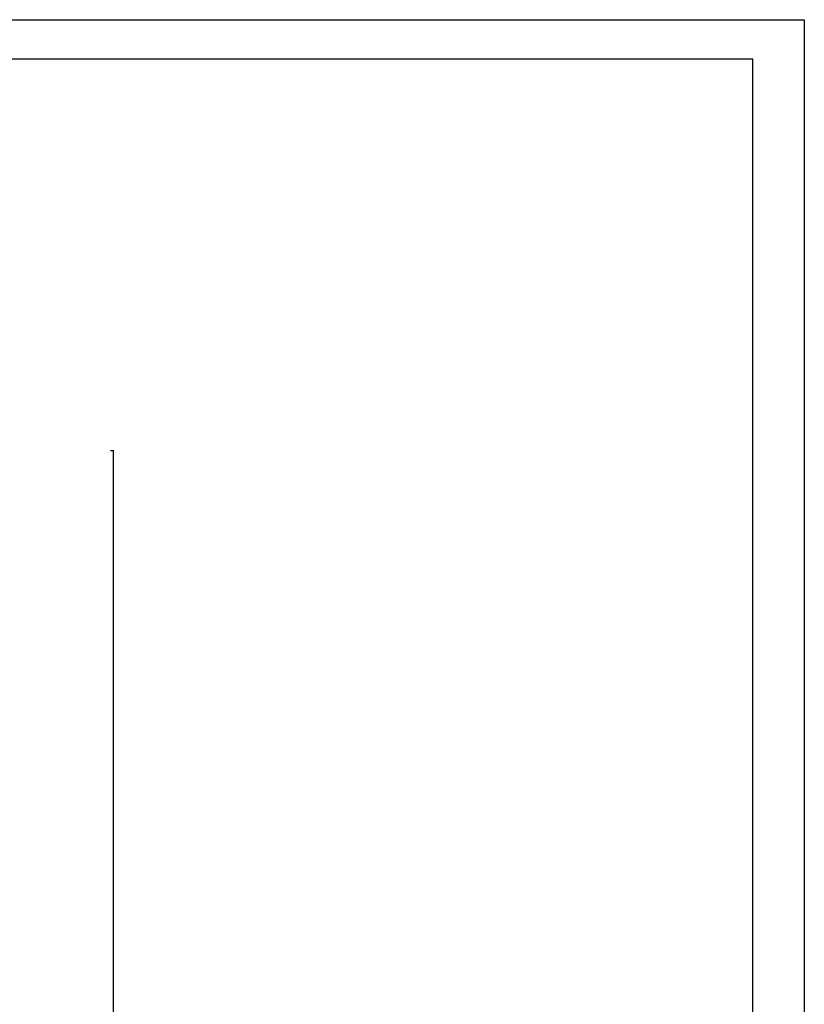
# Model space of a CAD drawing. Units: inches. Extents: x 0 to 4258, y 0 to 3769.
# Tile 30 of 30: x 4054 to 4258, y 3513 to 3769. Entities that reach past the tile are written whole.
import ezdxf

# ---------------------------------------------------------------- set-up
doc = ezdxf.new("R2010")
doc.units = ezdxf.units.IN
doc.header["$MEASUREMENT"] = 0
doc.layers.add('A-ANNO-DIMS', color=250, linetype='Continuous', lineweight=18)
doc.layers.add('A-ANNO-TTLB', color=250, linetype='Continuous', lineweight=25)
doc.styles.get("Standard").update_dxf_attribs({"font": 'arial.ttf'})
doc.dimstyles.get("Standard").update_dxf_attribs({"dimtxt": 7, "dimasz": 0.18, "dimexe": 0.18, "dimexo": 0.0625, "dimgap": 0.09, "dimtad": 0, "dimtih": 1, "dimtoh": 1, "dimzin": 0, "dimdsep": 46, "dimlunit": 3, "dimtxsty": 'Standard', "dimcen": 0.09, "dimadec": 0, "dimazin": 0, "dimtfac": 1, "dimtofl": 0, "dimtmove": 0, "dimatfit": 3, "dimfxl": 1, "dimtolj": 1, "dimtzin": 0, "dimarcsym": 0})

# ---------------------------------------------------------------- blocks, each defined once
blk = doc.blocks.new('*D26')
at = {"layer": 'A-ANNO-DIMS', "color": 0, "lineweight": -2, "transparency": 16777216}
for p, q in [((4077.41, 3656.79), (4078.27, 3656.79)), ((4078.09, 3656.61), (4078.09, 3329.69)), ((4078.09, 2995.47), (4078.09, 3322.39)), ((4077.41, 2995.29), (4078.27, 2995.29))]:
    blk.add_line(p, q, dxfattribs=at)
at = {"layer": 'A-ANNO-DIMS', "color": 0, "transparency": 16777216}
for points in [[(4078.06, 3656.61), (4078.12, 3656.61), (4078.09, 3656.79)], [(4078.06, 2995.47), (4078.12, 2995.47), (4078.09, 2995.29)]]:
    blk.add_solid(points, dxfattribs=at)
at = {"layer": 'Defpoints', "color": 0, "transparency": 16777216}
for p in [(4077.35, 3656.79), (4077.35, 2995.29), (4078.09, 2995.29)]:
    blk.add_point(p, dxfattribs=at)
at = {"layer": 'A-ANNO-DIMS', "color": 0, "transparency": 16777216, "insert": (4078.09, 3326.04), "char_height": 7, "attachment_point": 5}
blk.add_mtext("\\A1;55'", dxfattribs=at)

msp = doc.modelspace()

# ---------------------------------------------------------------- linework, layer by layer
at = {"layer": 'A-ANNO-TTLB'}
for p, q in [((3476.156, 3768.679), (4257.673, 3768.679)), ((4257.673, 3768.679), (4257.673, 2749.714)), ((4244.279, 3758.41), (3489.722, 3758.41)), ((4244.279, 2762.335), (4244.279, 3758.41))]:
    msp.add_line(p, q, dxfattribs=at)

# ---------------------------------------------------------------- dimensions: what is measured, and where the dimension line sits
at = {"layer": 'A-ANNO-DIMS'}
dim = msp.add_linear_dim(base=(4078.091, 2995.293), p1=(4077.346, 3656.793), p2=(4077.346, 2995.293), angle=90, text="55'", dimstyle='Standard', override={"dimclrd": 0, "dimclre": 0, "dimclrt": 0}, dxfattribs=at)
dim.commit()
dim.dimension.update_dxf_attribs({"geometry": '*D26', "text_midpoint": (4078.091, 3326.043)})

doc.saveas('drawing.dxf')
